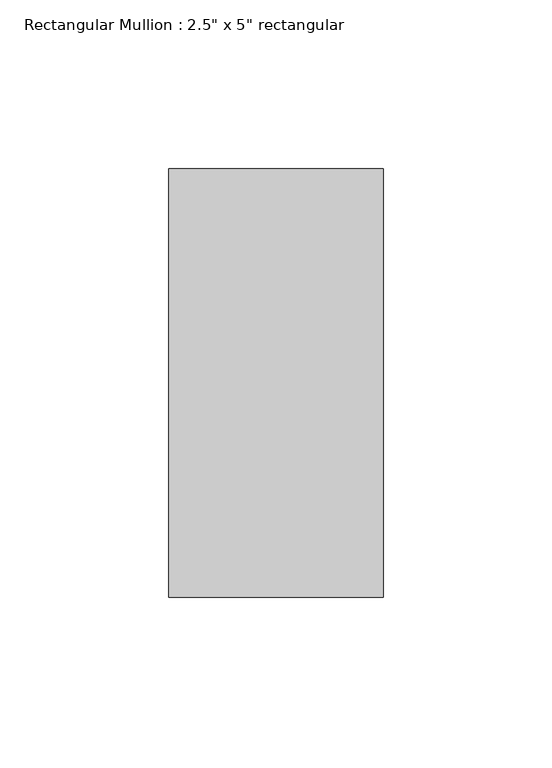
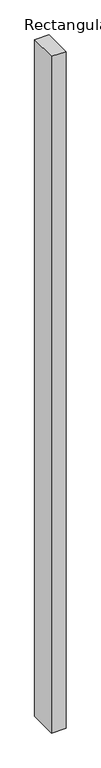
"""IFC4 building model written with IfcOpenShell, lengths in millimetres: member geometry."""

from ifc_helpers import new_model, si_unit, frame, origin, place, context, project, spatial, polyline, outline, extrude, source, transform, mapped, element, save


def member_c0191917(model_context):
    return source(origin(), model_context, "Body", "SweptSolid", [
        extrude(outline(polyline([(0.0, 63.5), (0.0, -63.5), (-63.5, -63.5), (-63.5, 63.5), (0.0, 63.5)])), frame((0.0, 0.0, -3116.9652567), z_axis=(0.0, 0.0, 1.0), x_axis=(1.0, 0.0, 0.0)), (0.0, 0.0, 1.0), 3116.9652567),
    ])


if __name__ == "__main__":
    model = new_model("IFC4")
    model_context = context("Model", 3, world=origin())
    ifc_project = project(units=[si_unit("LENGTHUNIT", "METRE", prefix="MILLI")], contexts=[model_context])
    site = spatial("IfcSite", under=ifc_project)
    building = spatial("IfcBuilding", under=site)
    placement = place(None, origin())
    member_shape = member_c0191917(model_context)
    element("IfcMember", 1, ObjectType="Rectangular Mullion : 2.5\" x 5\" rectangular", at=placement, inside=building, context=model_context, shape_type="MappedRepresentation", body=[
        mapped(member_shape, transform((0.0, 0.0, 0.0), x_axis=(1.0, 0.0, 0.0), y_axis=(0.0, 1.0, 0.0), z_axis=(0.0, 0.0, 1.0))),
    ])
    save(model, "model.ifc")

# Revit data of these elements
# Type "Rectangular Mullion : 2.5\" x 5\" rectangular"
#   built-in parameter 1007304 = 0.416667 (stored number, unit not read)
#   built-in parameter 1007301 = 0.104167 (stored number, unit not read)
#   built-in parameter 1007300 = 0.104167 (stored number, unit not read)
# Element 1 (IfcMember, "Rectangular Mullion : 2.5\" x 5\" rectangular")
#   Materials on its faces: "Iron, Ductile"
# Materials
#   "Iron, Ductile": class "Metal", colour RGB 0 0 0, transparency 0, Description = "Ductile cast iron", Cost = 0
